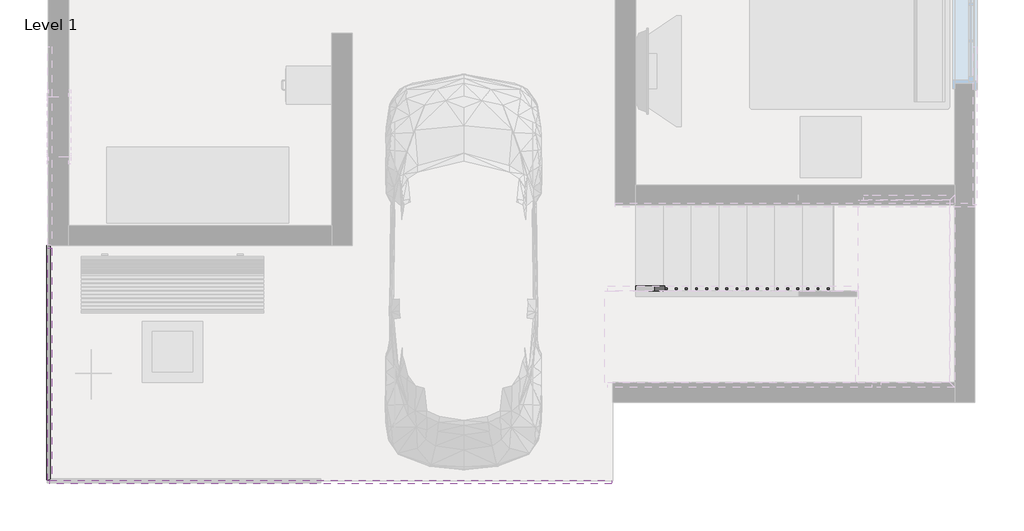
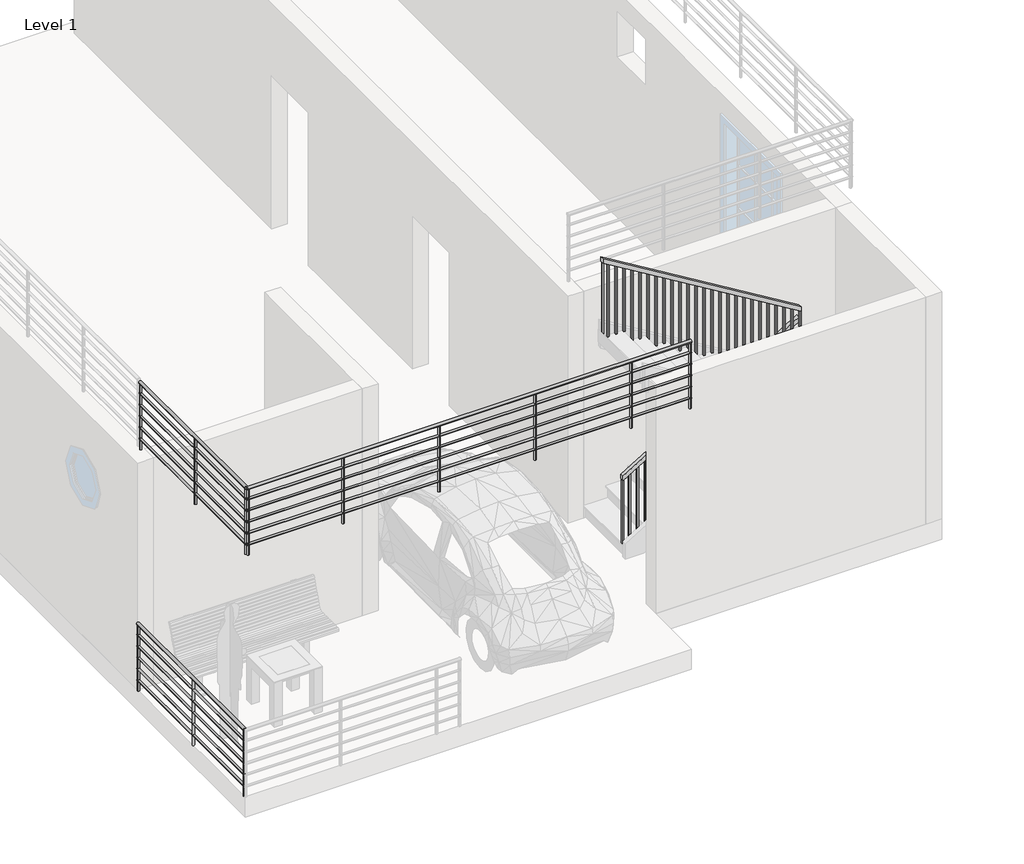
# One storey, part 2 of 4: 4 railings.
"""IFC4 building model written with IfcOpenShell, lengths in millimetres."""

from ifc_helpers import new_model, si_unit, point, frame, frame_2d, origin, origin_with_axes, place, context, project, spatial, polyline, circle_curve, trimmed, segment, composite_curve, outline, extrude, element, save

model = new_model("IFC4")

# Units and contexts
model_context = context("Model", 3, world=origin())
ifc_project = project(units=[si_unit("LENGTHUNIT", "METRE", prefix="MILLI")], contexts=[model_context])

# Site, building, storey
site = spatial("IfcSite", under=ifc_project)
building = spatial("IfcBuilding", under=site)
storey = spatial("IfcBuildingStorey", under=building, Name="Level 1", Elevation=0.0)

# Railings
placement = place(None, origin())
element("IfcRailing", 1, ObjectType="Handrail - Pipe", at=placement, inside=storey, context=model_context, shape_type="SweptSolid", body=[
    extrude(outline(composite_curve([segment(trimmed(circle_curve(frame_2d((4146.55, -14409.9389568)), 19.05), [point((4146.55, -14428.9889568))], [point((4146.55, -14390.8889568))], False, "CARTESIAN"), True, "CONTINUOUS"), segment(trimmed(circle_curve(frame_2d((4146.55, -14409.9389568)), 19.05), [point((4146.55, -14390.8889568))], [point((4146.55, -14428.9889568))], False, "CARTESIAN"), True, "CONTINUOUS")], self_intersect=False)), frame((0.0, 1290.5342758, 0.0), z_axis=(0.0, 1.0, 0.0), x_axis=(0.0, 0.0, 1.0)), (0.0, 0.0, 1.0), 2336.8),
    extrude(outline(composite_curve([segment(trimmed(circle_curve(frame_2d((4000.5, -14409.9389568)), 12.7), [point((4000.5, -14397.2389568))], [point((4000.5, -14422.6389568))], False, "CARTESIAN"), True, "CONTINUOUS"), segment(trimmed(circle_curve(frame_2d((4000.5, -14409.9389568)), 12.7), [point((4000.5, -14422.6389568))], [point((4000.5, -14397.2389568))], False, "CARTESIAN"), True, "CONTINUOUS")], self_intersect=False)), frame((0.0, 1290.5342758, 0.0), z_axis=(0.0, 1.0, 0.0), x_axis=(0.0, 0.0, 1.0)), (0.0, 0.0, 1.0), 2336.8),
    extrude(outline(composite_curve([segment(trimmed(circle_curve(frame_2d((3848.1, -14409.9389568)), 12.7), [point((3848.1, -14397.2389568))], [point((3848.1, -14422.6389568))], False, "CARTESIAN"), True, "CONTINUOUS"), segment(trimmed(circle_curve(frame_2d((3848.1, -14409.9389568)), 12.7), [point((3848.1, -14422.6389568))], [point((3848.1, -14397.2389568))], False, "CARTESIAN"), True, "CONTINUOUS")], self_intersect=False)), frame((0.0, 1290.5342758, 0.0), z_axis=(0.0, 1.0, 0.0), x_axis=(0.0, 0.0, 1.0)), (0.0, 0.0, 1.0), 2336.8),
    extrude(outline(composite_curve([segment(trimmed(circle_curve(frame_2d((3695.7, -14409.9389568)), 12.7), [point((3695.7, -14397.2389568))], [point((3695.7, -14422.6389568))], False, "CARTESIAN"), True, "CONTINUOUS"), segment(trimmed(circle_curve(frame_2d((3695.7, -14409.9389568)), 12.7), [point((3695.7, -14422.6389568))], [point((3695.7, -14397.2389568))], False, "CARTESIAN"), True, "CONTINUOUS")], self_intersect=False)), frame((0.0, 1290.5342758, 0.0), z_axis=(0.0, 1.0, 0.0), x_axis=(0.0, 0.0, 1.0)), (0.0, 0.0, 1.0), 2336.8),
    extrude(outline(composite_curve([segment(trimmed(circle_curve(frame_2d((3543.3, -14409.9389568)), 12.7), [point((3543.3, -14397.2389568))], [point((3543.3, -14422.6389568))], False, "CARTESIAN"), True, "CONTINUOUS"), segment(trimmed(circle_curve(frame_2d((3543.3, -14409.9389568)), 12.7), [point((3543.3, -14422.6389568))], [point((3543.3, -14397.2389568))], False, "CARTESIAN"), True, "CONTINUOUS")], self_intersect=False)), frame((0.0, 1290.5342758, 0.0), z_axis=(0.0, 1.0, 0.0), x_axis=(0.0, 0.0, 1.0)), (0.0, 0.0, 1.0), 2336.8),
    extrude(outline(composite_curve([segment(trimmed(circle_curve(frame_2d((3390.9, -14409.9389568)), 12.7), [point((3390.9, -14397.2389568))], [point((3390.9, -14422.6389568))], False, "CARTESIAN"), True, "CONTINUOUS"), segment(trimmed(circle_curve(frame_2d((3390.9, -14409.9389568)), 12.7), [point((3390.9, -14422.6389568))], [point((3390.9, -14397.2389568))], False, "CARTESIAN"), True, "CONTINUOUS")], self_intersect=False)), frame((0.0, 1290.5342758, 0.0), z_axis=(0.0, 1.0, 0.0), x_axis=(0.0, 0.0, 1.0)), (0.0, 0.0, 1.0), 2336.8),
    extrude(outline(composite_curve([segment(trimmed(circle_curve(frame_2d((-14409.9389568, 2408.1342758)), 12.7), [point((-14397.2389568, 2408.1342758))], [point((-14422.6389568, 2408.1342758))], False, "CARTESIAN"), True, "CONTINUOUS"), segment(trimmed(circle_curve(frame_2d((-14409.9389568, 2408.1342758)), 12.7), [point((-14422.6389568, 2408.1342758))], [point((-14397.2389568, 2408.1342758))], False, "CARTESIAN"), True, "CONTINUOUS")], self_intersect=False)), frame((0.0, 0.0, 3251.2), z_axis=(0.0, 0.0, 1.0), x_axis=(1.0, 0.0, 0.0)), (0.0, 0.0, 1.0), 876.3),
    extrude(outline(composite_curve([segment(trimmed(circle_curve(frame_2d((-14409.9389568, 1303.2342758)), 12.7), [point((-14397.2389568, 1303.2342758))], [point((-14422.6389568, 1303.2342758))], False, "CARTESIAN"), True, "CONTINUOUS"), segment(trimmed(circle_curve(frame_2d((-14409.9389568, 1303.2342758)), 12.7), [point((-14422.6389568, 1303.2342758))], [point((-14397.2389568, 1303.2342758))], False, "CARTESIAN"), True, "CONTINUOUS")], self_intersect=False)), frame((0.0, 0.0, 3251.2), z_axis=(0.0, 0.0, 1.0), x_axis=(1.0, 0.0, 0.0)), (0.0, 0.0, 1.0), 876.3),
    extrude(outline(composite_curve([segment(trimmed(circle_curve(frame_2d((-14409.9389568, 3614.6342758)), 12.7), [point((-14397.2389568, 3614.6342758))], [point((-14422.6389568, 3614.6342758))], False, "CARTESIAN"), True, "CONTINUOUS"), segment(trimmed(circle_curve(frame_2d((-14409.9389568, 3614.6342758)), 12.7), [point((-14422.6389568, 3614.6342758))], [point((-14397.2389568, 3614.6342758))], False, "CARTESIAN"), True, "CONTINUOUS")], self_intersect=False)), frame((0.0, 0.0, 3251.2), z_axis=(0.0, 0.0, 1.0), x_axis=(1.0, 0.0, 0.0)), (0.0, 0.0, 1.0), 876.3),
])
element("IfcRailing", 2, ObjectType="Handrail - Pipe", at=placement, inside=storey, context=model_context, shape_type="SweptSolid", body=[
    extrude(outline(composite_curve([segment(trimmed(circle_curve(frame_2d((895.35, -14422.6389568)), 19.05), [point((895.35, -14441.6889568))], [point((895.35, -14403.5889568))], False, "CARTESIAN"), True, "CONTINUOUS"), segment(trimmed(circle_curve(frame_2d((895.35, -14422.6389568)), 19.05), [point((895.35, -14403.5889568))], [point((895.35, -14441.6889568))], False, "CARTESIAN"), True, "CONTINUOUS")], self_intersect=False)), frame((0.0, 1303.2342758, 0.0), z_axis=(0.0, 1.0, 0.0), x_axis=(0.0, 0.0, 1.0)), (0.0, 0.0, 1.0), 2349.5),
    extrude(outline(composite_curve([segment(trimmed(circle_curve(frame_2d((749.3, -14422.6389568)), 12.7), [point((749.3, -14409.9389568))], [point((749.3, -14435.3389568))], False, "CARTESIAN"), True, "CONTINUOUS"), segment(trimmed(circle_curve(frame_2d((749.3, -14422.6389568)), 12.7), [point((749.3, -14435.3389568))], [point((749.3, -14409.9389568))], False, "CARTESIAN"), True, "CONTINUOUS")], self_intersect=False)), frame((0.0, 1303.2342758, 0.0), z_axis=(0.0, 1.0, 0.0), x_axis=(0.0, 0.0, 1.0)), (0.0, 0.0, 1.0), 2349.5),
    extrude(outline(composite_curve([segment(trimmed(circle_curve(frame_2d((596.9, -14422.6389568)), 12.7), [point((596.9, -14409.9389568))], [point((596.9, -14435.3389568))], False, "CARTESIAN"), True, "CONTINUOUS"), segment(trimmed(circle_curve(frame_2d((596.9, -14422.6389568)), 12.7), [point((596.9, -14435.3389568))], [point((596.9, -14409.9389568))], False, "CARTESIAN"), True, "CONTINUOUS")], self_intersect=False)), frame((0.0, 1303.2342758, 0.0), z_axis=(0.0, 1.0, 0.0), x_axis=(0.0, 0.0, 1.0)), (0.0, 0.0, 1.0), 2349.5),
    extrude(outline(composite_curve([segment(trimmed(circle_curve(frame_2d((444.5, -14422.6389568)), 12.7), [point((444.5, -14409.9389568))], [point((444.5, -14435.3389568))], False, "CARTESIAN"), True, "CONTINUOUS"), segment(trimmed(circle_curve(frame_2d((444.5, -14422.6389568)), 12.7), [point((444.5, -14435.3389568))], [point((444.5, -14409.9389568))], False, "CARTESIAN"), True, "CONTINUOUS")], self_intersect=False)), frame((0.0, 1303.2342758, 0.0), z_axis=(0.0, 1.0, 0.0), x_axis=(0.0, 0.0, 1.0)), (0.0, 0.0, 1.0), 2349.5),
    extrude(outline(composite_curve([segment(trimmed(circle_curve(frame_2d((292.1, -14422.6389568)), 12.7), [point((292.1, -14409.9389568))], [point((292.1, -14435.3389568))], False, "CARTESIAN"), True, "CONTINUOUS"), segment(trimmed(circle_curve(frame_2d((292.1, -14422.6389568)), 12.7), [point((292.1, -14435.3389568))], [point((292.1, -14409.9389568))], False, "CARTESIAN"), True, "CONTINUOUS")], self_intersect=False)), frame((0.0, 1303.2342758, 0.0), z_axis=(0.0, 1.0, 0.0), x_axis=(0.0, 0.0, 1.0)), (0.0, 0.0, 1.0), 2349.5),
    extrude(outline(composite_curve([segment(trimmed(circle_curve(frame_2d((139.7, -14422.6389568)), 12.7), [point((139.7, -14409.9389568))], [point((139.7, -14435.3389568))], False, "CARTESIAN"), True, "CONTINUOUS"), segment(trimmed(circle_curve(frame_2d((139.7, -14422.6389568)), 12.7), [point((139.7, -14435.3389568))], [point((139.7, -14409.9389568))], False, "CARTESIAN"), True, "CONTINUOUS")], self_intersect=False)), frame((0.0, 1303.2342758, 0.0), z_axis=(0.0, 1.0, 0.0), x_axis=(0.0, 0.0, 1.0)), (0.0, 0.0, 1.0), 2349.5),
    extrude(outline(composite_curve([segment(trimmed(circle_curve(frame_2d((-14422.6389568, 2433.5342758)), 12.7), [point((-14409.9389568, 2433.5342758))], [point((-14435.3389568, 2433.5342758))], False, "CARTESIAN"), True, "CONTINUOUS"), segment(trimmed(circle_curve(frame_2d((-14422.6389568, 2433.5342758)), 12.7), [point((-14435.3389568, 2433.5342758))], [point((-14409.9389568, 2433.5342758))], False, "CARTESIAN"), True, "CONTINUOUS")], self_intersect=False)), origin_with_axes(), (0.0, 0.0, 1.0), 876.3),
    extrude(outline(composite_curve([segment(trimmed(circle_curve(frame_2d((-14422.6389568, 1315.9342758)), 12.7), [point((-14409.9389568, 1315.9342758))], [point((-14435.3389568, 1315.9342758))], False, "CARTESIAN"), True, "CONTINUOUS"), segment(trimmed(circle_curve(frame_2d((-14422.6389568, 1315.9342758)), 12.7), [point((-14435.3389568, 1315.9342758))], [point((-14409.9389568, 1315.9342758))], False, "CARTESIAN"), True, "CONTINUOUS")], self_intersect=False)), origin_with_axes(), (0.0, 0.0, 1.0), 876.3),
    extrude(outline(composite_curve([segment(trimmed(circle_curve(frame_2d((-14422.6389568, 3640.0342758)), 12.7), [point((-14409.9389568, 3640.0342758))], [point((-14435.3389568, 3640.0342758))], False, "CARTESIAN"), True, "CONTINUOUS"), segment(trimmed(circle_curve(frame_2d((-14422.6389568, 3640.0342758)), 12.7), [point((-14435.3389568, 3640.0342758))], [point((-14409.9389568, 3640.0342758))], False, "CARTESIAN"), True, "CONTINUOUS")], self_intersect=False)), origin_with_axes(), (0.0, 0.0, 1.0), 876.3),
])
element("IfcRailing", 3, ObjectType="Handrail - Pipe", at=placement, inside=storey, context=model_context, shape_type="SweptSolid", body=[
    extrude(outline(composite_curve([segment(trimmed(circle_curve(frame_2d((1277.8342758, 4146.55)), 19.05), [point((1258.7842758, 4146.55))], [point((1296.8842758, 4146.55))], False, "CARTESIAN"), True, "CONTINUOUS"), segment(trimmed(circle_curve(frame_2d((1277.8342758, 4146.55)), 19.05), [point((1296.8842758, 4146.55))], [point((1258.7842758, 4146.55))], False, "CARTESIAN"), True, "CONTINUOUS")], self_intersect=False)), frame((-14409.9389568, 0.0, 0.0), z_axis=(1.0, 0.0, 0.0), x_axis=(0.0, 1.0, 0.0)), (0.0, 0.0, 1.0), 5638.8),
    extrude(outline(composite_curve([segment(trimmed(circle_curve(frame_2d((1277.8342758, 4000.5)), 12.7), [point((1290.5342758, 4000.5))], [point((1265.1342758, 4000.5))], False, "CARTESIAN"), True, "CONTINUOUS"), segment(trimmed(circle_curve(frame_2d((1277.8342758, 4000.5)), 12.7), [point((1265.1342758, 4000.5))], [point((1290.5342758, 4000.5))], False, "CARTESIAN"), True, "CONTINUOUS")], self_intersect=False)), frame((-14409.9389568, 0.0, 0.0), z_axis=(1.0, 0.0, 0.0), x_axis=(0.0, 1.0, 0.0)), (0.0, 0.0, 1.0), 5638.8),
    extrude(outline(composite_curve([segment(trimmed(circle_curve(frame_2d((1277.8342758, 3848.1)), 12.7), [point((1290.5342758, 3848.1))], [point((1265.1342758, 3848.1))], False, "CARTESIAN"), True, "CONTINUOUS"), segment(trimmed(circle_curve(frame_2d((1277.8342758, 3848.1)), 12.7), [point((1265.1342758, 3848.1))], [point((1290.5342758, 3848.1))], False, "CARTESIAN"), True, "CONTINUOUS")], self_intersect=False)), frame((-14409.9389568, 0.0, 0.0), z_axis=(1.0, 0.0, 0.0), x_axis=(0.0, 1.0, 0.0)), (0.0, 0.0, 1.0), 5638.8),
    extrude(outline(composite_curve([segment(trimmed(circle_curve(frame_2d((1277.8342758, 3695.7)), 12.7), [point((1290.5342758, 3695.7))], [point((1265.1342758, 3695.7))], False, "CARTESIAN"), True, "CONTINUOUS"), segment(trimmed(circle_curve(frame_2d((1277.8342758, 3695.7)), 12.7), [point((1265.1342758, 3695.7))], [point((1290.5342758, 3695.7))], False, "CARTESIAN"), True, "CONTINUOUS")], self_intersect=False)), frame((-14409.9389568, 0.0, 0.0), z_axis=(1.0, 0.0, 0.0), x_axis=(0.0, 1.0, 0.0)), (0.0, 0.0, 1.0), 5638.8),
    extrude(outline(composite_curve([segment(trimmed(circle_curve(frame_2d((1277.8342758, 3543.3)), 12.7), [point((1290.5342758, 3543.3))], [point((1265.1342758, 3543.3))], False, "CARTESIAN"), True, "CONTINUOUS"), segment(trimmed(circle_curve(frame_2d((1277.8342758, 3543.3)), 12.7), [point((1265.1342758, 3543.3))], [point((1290.5342758, 3543.3))], False, "CARTESIAN"), True, "CONTINUOUS")], self_intersect=False)), frame((-14409.9389568, 0.0, 0.0), z_axis=(1.0, 0.0, 0.0), x_axis=(0.0, 1.0, 0.0)), (0.0, 0.0, 1.0), 5638.8),
    extrude(outline(composite_curve([segment(trimmed(circle_curve(frame_2d((1277.8342758, 3390.9)), 12.7), [point((1290.5342758, 3390.9))], [point((1265.1342758, 3390.9))], False, "CARTESIAN"), True, "CONTINUOUS"), segment(trimmed(circle_curve(frame_2d((1277.8342758, 3390.9)), 12.7), [point((1265.1342758, 3390.9))], [point((1290.5342758, 3390.9))], False, "CARTESIAN"), True, "CONTINUOUS")], self_intersect=False)), frame((-14409.9389568, 0.0, 0.0), z_axis=(1.0, 0.0, 0.0), x_axis=(0.0, 1.0, 0.0)), (0.0, 0.0, 1.0), 5638.8),
    extrude(outline(composite_curve([segment(trimmed(circle_curve(frame_2d((-9533.1389568, 1277.8342758)), 12.7), [point((-9533.1389568, 1290.5342758))], [point((-9533.1389568, 1265.1342758))], False, "CARTESIAN"), True, "CONTINUOUS"), segment(trimmed(circle_curve(frame_2d((-9533.1389568, 1277.8342758)), 12.7), [point((-9533.1389568, 1265.1342758))], [point((-9533.1389568, 1290.5342758))], False, "CARTESIAN"), True, "CONTINUOUS")], self_intersect=False)), frame((0.0, 0.0, 3251.2), z_axis=(0.0, 0.0, 1.0), x_axis=(1.0, 0.0, 0.0)), (0.0, 0.0, 1.0), 876.3),
    extrude(outline(composite_curve([segment(trimmed(circle_curve(frame_2d((-10752.3389568, 1277.8342758)), 12.7), [point((-10752.3389568, 1290.5342758))], [point((-10752.3389568, 1265.1342758))], False, "CARTESIAN"), True, "CONTINUOUS"), segment(trimmed(circle_curve(frame_2d((-10752.3389568, 1277.8342758)), 12.7), [point((-10752.3389568, 1265.1342758))], [point((-10752.3389568, 1290.5342758))], False, "CARTESIAN"), True, "CONTINUOUS")], self_intersect=False)), frame((0.0, 0.0, 3251.2), z_axis=(0.0, 0.0, 1.0), x_axis=(1.0, 0.0, 0.0)), (0.0, 0.0, 1.0), 876.3),
    extrude(outline(composite_curve([segment(trimmed(circle_curve(frame_2d((-11971.5389568, 1277.8342758)), 12.7), [point((-11971.5389568, 1290.5342758))], [point((-11971.5389568, 1265.1342758))], False, "CARTESIAN"), True, "CONTINUOUS"), segment(trimmed(circle_curve(frame_2d((-11971.5389568, 1277.8342758)), 12.7), [point((-11971.5389568, 1265.1342758))], [point((-11971.5389568, 1290.5342758))], False, "CARTESIAN"), True, "CONTINUOUS")], self_intersect=False)), frame((0.0, 0.0, 3251.2), z_axis=(0.0, 0.0, 1.0), x_axis=(1.0, 0.0, 0.0)), (0.0, 0.0, 1.0), 876.3),
    extrude(outline(composite_curve([segment(trimmed(circle_curve(frame_2d((-13190.7389568, 1277.8342758)), 12.7), [point((-13190.7389568, 1290.5342758))], [point((-13190.7389568, 1265.1342758))], False, "CARTESIAN"), True, "CONTINUOUS"), segment(trimmed(circle_curve(frame_2d((-13190.7389568, 1277.8342758)), 12.7), [point((-13190.7389568, 1265.1342758))], [point((-13190.7389568, 1290.5342758))], False, "CARTESIAN"), True, "CONTINUOUS")], self_intersect=False)), frame((0.0, 0.0, 3251.2), z_axis=(0.0, 0.0, 1.0), x_axis=(1.0, 0.0, 0.0)), (0.0, 0.0, 1.0), 876.3),
    extrude(outline(composite_curve([segment(trimmed(circle_curve(frame_2d((-8783.8389568, 1277.8342758)), 12.7), [point((-8783.8389568, 1290.5342758))], [point((-8783.8389568, 1265.1342758))], False, "CARTESIAN"), True, "CONTINUOUS"), segment(trimmed(circle_curve(frame_2d((-8783.8389568, 1277.8342758)), 12.7), [point((-8783.8389568, 1265.1342758))], [point((-8783.8389568, 1290.5342758))], False, "CARTESIAN"), True, "CONTINUOUS")], self_intersect=False)), frame((0.0, 0.0, 3251.2), z_axis=(0.0, 0.0, 1.0), x_axis=(1.0, 0.0, 0.0)), (0.0, 0.0, 1.0), 876.3),
    extrude(outline(composite_curve([segment(trimmed(circle_curve(frame_2d((-14397.2389568, 1277.8342758)), 12.7), [point((-14397.2389568, 1290.5342758))], [point((-14397.2389568, 1265.1342758))], False, "CARTESIAN"), True, "CONTINUOUS"), segment(trimmed(circle_curve(frame_2d((-14397.2389568, 1277.8342758)), 12.7), [point((-14397.2389568, 1265.1342758))], [point((-14397.2389568, 1290.5342758))], False, "CARTESIAN"), True, "CONTINUOUS")], self_intersect=False)), frame((0.0, 0.0, 3251.2), z_axis=(0.0, 0.0, 1.0), x_axis=(1.0, 0.0, 0.0)), (0.0, 0.0, 1.0), 876.3),
])
element("IfcRailing", 4, ObjectType="Handrail - Rectangular", at=placement, inside=storey, context=model_context, shape_type="SweptSolid", body=[
    extrude(outline(polyline([(1083.7333333, -8529.8389568), (1024.3318731, -8529.8389568), (2378.9985397, -6294.6389568), (2438.4, -6294.6389568), (1083.7333333, -8529.8389568)])), frame((0.0, 3195.5342758, 0.0), z_axis=(0.0, 1.0, 0.0), x_axis=(0.0, 0.0, 1.0)), (0.0, 0.0, 1.0), 50.8),
    extrude(outline(polyline([(2548.3318731, -6294.6389568), (2607.7333333, -6294.6389568), (4131.7333333, -8809.2389568), (4072.3318731, -8809.2389568), (2548.3318731, -6294.6389568)])), frame((0.0, 3144.7342758, 0.0), z_axis=(0.0, 1.0, 0.0), x_axis=(0.0, 0.0, 1.0)), (0.0, 0.0, 1.0), 50.8),
    extrude(outline(polyline([(4020.3773276, -8723.5139568), (4031.9227822, -8742.5639568), (3048.0, -8742.5639568), (3048.0, -8723.5139568), (4020.3773276, -8723.5139568)])), frame((0.0, 3160.6092758, 0.0), z_axis=(0.0, 1.0, 0.0), x_axis=(0.0, 0.0, 1.0)), (0.0, 0.0, 1.0), 19.05),
    extrude(outline(polyline([(3958.80157, -8621.9139568), (3970.3470246, -8640.9639568), (3048.0, -8640.9639568), (3048.0, -8621.9139568), (3958.80157, -8621.9139568)])), frame((0.0, 3160.6092758, 0.0), z_axis=(0.0, 1.0, 0.0), x_axis=(0.0, 0.0, 1.0)), (0.0, 0.0, 1.0), 19.05),
    extrude(outline(polyline([(3897.2258125, -8520.3139568), (3908.771267, -8539.3639568), (3048.0, -8539.3639568), (3048.0, -8520.3139568), (3897.2258125, -8520.3139568)])), frame((0.0, 3160.6092758, 0.0), z_axis=(0.0, 1.0, 0.0), x_axis=(0.0, 0.0, 1.0)), (0.0, 0.0, 1.0), 19.05),
    extrude(outline(polyline([(3835.6500549, -8418.7139568), (3847.1955094, -8437.7639568), (2878.6666667, -8437.7639568), (2878.6666667, -8418.7139568), (3835.6500549, -8418.7139568)])), frame((0.0, 3160.6092758, 0.0), z_axis=(0.0, 1.0, 0.0), x_axis=(0.0, 0.0, 1.0)), (0.0, 0.0, 1.0), 19.05),
    extrude(outline(polyline([(3774.0742973, -8317.1139568), (3785.6197519, -8336.1639568), (2878.6666667, -8336.1639568), (2878.6666667, -8317.1139568), (3774.0742973, -8317.1139568)])), frame((0.0, 3160.6092758, 0.0), z_axis=(0.0, 1.0, 0.0), x_axis=(0.0, 0.0, 1.0)), (0.0, 0.0, 1.0), 19.05),
    extrude(outline(polyline([(3712.4985397, -8215.5139568), (3724.0439943, -8234.5639568), (2709.3333333, -8234.5639568), (2709.3333333, -8215.5139568), (3712.4985397, -8215.5139568)])), frame((0.0, 3160.6092758, 0.0), z_axis=(0.0, 1.0, 0.0), x_axis=(0.0, 0.0, 1.0)), (0.0, 0.0, 1.0), 19.05),
    extrude(outline(polyline([(3650.9227822, -8113.9139568), (3662.4682367, -8132.9639568), (2709.3333333, -8132.9639568), (2709.3333333, -8113.9139568), (3650.9227822, -8113.9139568)])), frame((0.0, 3160.6092758, 0.0), z_axis=(0.0, 1.0, 0.0), x_axis=(0.0, 0.0, 1.0)), (0.0, 0.0, 1.0), 19.05),
    extrude(outline(polyline([(3589.3470246, -8012.3139568), (3600.8924791, -8031.3639568), (2709.3333333, -8031.3639568), (2709.3333333, -8012.3139568), (3589.3470246, -8012.3139568)])), frame((0.0, 3160.6092758, 0.0), z_axis=(0.0, 1.0, 0.0), x_axis=(0.0, 0.0, 1.0)), (0.0, 0.0, 1.0), 19.05),
    extrude(outline(polyline([(3527.771267, -7910.7139568), (3539.3167216, -7929.7639568), (2540.0, -7929.7639568), (2540.0, -7910.7139568), (3527.771267, -7910.7139568)])), frame((0.0, 3160.6092758, 0.0), z_axis=(0.0, 1.0, 0.0), x_axis=(0.0, 0.0, 1.0)), (0.0, 0.0, 1.0), 19.05),
    extrude(outline(polyline([(3466.1955094, -7809.1139568), (3477.740964, -7828.1639568), (2540.0, -7828.1639568), (2540.0, -7809.1139568), (3466.1955094, -7809.1139568)])), frame((0.0, 3160.6092758, 0.0), z_axis=(0.0, 1.0, 0.0), x_axis=(0.0, 0.0, 1.0)), (0.0, 0.0, 1.0), 19.05),
    extrude(outline(polyline([(3404.6197519, -7707.5139568), (3416.1652064, -7726.5639568), (2540.0, -7726.5639568), (2540.0, -7707.5139568), (3404.6197519, -7707.5139568)])), frame((0.0, 3160.6092758, 0.0), z_axis=(0.0, 1.0, 0.0), x_axis=(0.0, 0.0, 1.0)), (0.0, 0.0, 1.0), 19.05),
    extrude(outline(polyline([(3343.0439943, -7605.9139568), (3354.5894488, -7624.9639568), (2370.6666667, -7624.9639568), (2370.6666667, -7605.9139568), (3343.0439943, -7605.9139568)])), frame((0.0, 3160.6092758, 0.0), z_axis=(0.0, 1.0, 0.0), x_axis=(0.0, 0.0, 1.0)), (0.0, 0.0, 1.0), 19.05),
    extrude(outline(polyline([(3281.4682367, -7504.3139568), (3293.0136913, -7523.3639568), (2370.6666667, -7523.3639568), (2370.6666667, -7504.3139568), (3281.4682367, -7504.3139568)])), frame((0.0, 3160.6092758, 0.0), z_axis=(0.0, 1.0, 0.0), x_axis=(0.0, 0.0, 1.0)), (0.0, 0.0, 1.0), 19.05),
    extrude(outline(polyline([(3219.8924791, -7402.7139568), (3231.4379337, -7421.7639568), (2370.6666667, -7421.7639568), (2370.6666667, -7402.7139568), (3219.8924791, -7402.7139568)])), frame((0.0, 3160.6092758, 0.0), z_axis=(0.0, 1.0, 0.0), x_axis=(0.0, 0.0, 1.0)), (0.0, 0.0, 1.0), 19.05),
    extrude(outline(polyline([(3158.3167216, -7301.1139568), (3169.8621761, -7320.1639568), (2201.3333333, -7320.1639568), (2201.3333333, -7301.1139568), (3158.3167216, -7301.1139568)])), frame((0.0, 3160.6092758, 0.0), z_axis=(0.0, 1.0, 0.0), x_axis=(0.0, 0.0, 1.0)), (0.0, 0.0, 1.0), 19.05),
    extrude(outline(polyline([(3096.740964, -7199.5139568), (3108.2864185, -7218.5639568), (2201.3333333, -7218.5639568), (2201.3333333, -7199.5139568), (3096.740964, -7199.5139568)])), frame((0.0, 3160.6092758, 0.0), z_axis=(0.0, 1.0, 0.0), x_axis=(0.0, 0.0, 1.0)), (0.0, 0.0, 1.0), 19.05),
    extrude(outline(polyline([(3035.1652064, -7097.9139568), (3046.710661, -7116.9639568), (2032.0, -7116.9639568), (2032.0, -7097.9139568), (3035.1652064, -7097.9139568)])), frame((0.0, 3160.6092758, 0.0), z_axis=(0.0, 1.0, 0.0), x_axis=(0.0, 0.0, 1.0)), (0.0, 0.0, 1.0), 19.05),
    extrude(outline(polyline([(2973.5894488, -6996.3139568), (2985.1349034, -7015.3639568), (2032.0, -7015.3639568), (2032.0, -6996.3139568), (2973.5894488, -6996.3139568)])), frame((0.0, 3160.6092758, 0.0), z_axis=(0.0, 1.0, 0.0), x_axis=(0.0, 0.0, 1.0)), (0.0, 0.0, 1.0), 19.05),
    extrude(outline(polyline([(2912.0136913, -6894.7139568), (2923.5591458, -6913.7639568), (2032.0, -6913.7639568), (2032.0, -6894.7139568), (2912.0136913, -6894.7139568)])), frame((0.0, 3160.6092758, 0.0), z_axis=(0.0, 1.0, 0.0), x_axis=(0.0, 0.0, 1.0)), (0.0, 0.0, 1.0), 19.05),
    extrude(outline(polyline([(2850.4379337, -6793.1139568), (2861.9833882, -6812.1639568), (1862.6666667, -6812.1639568), (1862.6666667, -6793.1139568), (2850.4379337, -6793.1139568)])), frame((0.0, 3160.6092758, 0.0), z_axis=(0.0, 1.0, 0.0), x_axis=(0.0, 0.0, 1.0)), (0.0, 0.0, 1.0), 19.05),
    extrude(outline(polyline([(2788.8621761, -6691.5139568), (2800.4076307, -6710.5639568), (1862.6666667, -6710.5639568), (1862.6666667, -6691.5139568), (2788.8621761, -6691.5139568)])), frame((0.0, 3160.6092758, 0.0), z_axis=(0.0, 1.0, 0.0), x_axis=(0.0, 0.0, 1.0)), (0.0, 0.0, 1.0), 19.05),
    extrude(outline(polyline([(2727.2864185, -6589.9139568), (2738.8318731, -6608.9639568), (1862.6666667, -6608.9639568), (1862.6666667, -6589.9139568), (2727.2864185, -6589.9139568)])), frame((0.0, 3160.6092758, 0.0), z_axis=(0.0, 1.0, 0.0), x_axis=(0.0, 0.0, 1.0)), (0.0, 0.0, 1.0), 19.05),
    extrude(outline(polyline([(2665.710661, -6488.3139568), (2677.2561155, -6507.3639568), (1693.3333333, -6507.3639568), (1693.3333333, -6488.3139568), (2665.710661, -6488.3139568)])), frame((0.0, 3160.6092758, 0.0), z_axis=(0.0, 1.0, 0.0), x_axis=(0.0, 0.0, 1.0)), (0.0, 0.0, 1.0), 19.05),
    extrude(outline(polyline([(2604.1349034, -6386.7139568), (2615.6803579, -6405.7639568), (1693.3333333, -6405.7639568), (1693.3333333, -6386.7139568), (2604.1349034, -6386.7139568)])), frame((0.0, 3160.6092758, 0.0), z_axis=(0.0, 1.0, 0.0), x_axis=(0.0, 0.0, 1.0)), (0.0, 0.0, 1.0), 19.05),
    extrude(outline(polyline([(2323.1955094, -6386.7139568), (2311.6500549, -6405.7639568), (1354.6666667, -6405.7639568), (1354.6666667, -6386.7139568), (2323.1955094, -6386.7139568)])), frame((0.0, 3211.4092758, 0.0), z_axis=(0.0, 1.0, 0.0), x_axis=(0.0, 0.0, 1.0)), (0.0, 0.0, 1.0), 19.05),
    extrude(outline(polyline([(2261.6197519, -6488.3139568), (2250.0742973, -6507.3639568), (1354.6666667, -6507.3639568), (1354.6666667, -6488.3139568), (2261.6197519, -6488.3139568)])), frame((0.0, 3211.4092758, 0.0), z_axis=(0.0, 1.0, 0.0), x_axis=(0.0, 0.0, 1.0)), (0.0, 0.0, 1.0), 19.05),
    extrude(outline(polyline([(2200.0439943, -6589.9139568), (2188.4985397, -6608.9639568), (1185.3333333, -6608.9639568), (1185.3333333, -6589.9139568), (2200.0439943, -6589.9139568)])), frame((0.0, 3211.4092758, 0.0), z_axis=(0.0, 1.0, 0.0), x_axis=(0.0, 0.0, 1.0)), (0.0, 0.0, 1.0), 19.05),
    extrude(outline(polyline([(2138.4682367, -6691.5139568), (2126.9227822, -6710.5639568), (1185.3333333, -6710.5639568), (1185.3333333, -6691.5139568), (2138.4682367, -6691.5139568)])), frame((0.0, 3211.4092758, 0.0), z_axis=(0.0, 1.0, 0.0), x_axis=(0.0, 0.0, 1.0)), (0.0, 0.0, 1.0), 19.05),
    extrude(outline(polyline([(2076.8924791, -6793.1139568), (2065.3470246, -6812.1639568), (1185.3333333, -6812.1639568), (1185.3333333, -6793.1139568), (2076.8924791, -6793.1139568)])), frame((0.0, 3211.4092758, 0.0), z_axis=(0.0, 1.0, 0.0), x_axis=(0.0, 0.0, 1.0)), (0.0, 0.0, 1.0), 19.05),
    extrude(outline(polyline([(2015.3167216, -6894.7139568), (2003.771267, -6913.7639568), (1016.0, -6913.7639568), (1016.0, -6894.7139568), (2015.3167216, -6894.7139568)])), frame((0.0, 3211.4092758, 0.0), z_axis=(0.0, 1.0, 0.0), x_axis=(0.0, 0.0, 1.0)), (0.0, 0.0, 1.0), 19.05),
    extrude(outline(polyline([(1953.740964, -6996.3139568), (1942.1955094, -7015.3639568), (1016.0, -7015.3639568), (1016.0, -6996.3139568), (1953.740964, -6996.3139568)])), frame((0.0, 3211.4092758, 0.0), z_axis=(0.0, 1.0, 0.0), x_axis=(0.0, 0.0, 1.0)), (0.0, 0.0, 1.0), 19.05),
    extrude(outline(polyline([(1892.1652064, -7097.9139568), (1880.6197519, -7116.9639568), (1016.0, -7116.9639568), (1016.0, -7097.9139568), (1892.1652064, -7097.9139568)])), frame((0.0, 3211.4092758, 0.0), z_axis=(0.0, 1.0, 0.0), x_axis=(0.0, 0.0, 1.0)), (0.0, 0.0, 1.0), 19.05),
    extrude(outline(polyline([(1830.5894488, -7199.5139568), (1819.0439943, -7218.5639568), (846.6666667, -7218.5639568), (846.6666667, -7199.5139568), (1830.5894488, -7199.5139568)])), frame((0.0, 3211.4092758, 0.0), z_axis=(0.0, 1.0, 0.0), x_axis=(0.0, 0.0, 1.0)), (0.0, 0.0, 1.0), 19.05),
    extrude(outline(polyline([(1769.0136913, -7301.1139568), (1757.4682367, -7320.1639568), (846.6666667, -7320.1639568), (846.6666667, -7301.1139568), (1769.0136913, -7301.1139568)])), frame((0.0, 3211.4092758, 0.0), z_axis=(0.0, 1.0, 0.0), x_axis=(0.0, 0.0, 1.0)), (0.0, 0.0, 1.0), 19.05),
    extrude(outline(polyline([(1707.4379337, -7402.7139568), (1695.8924791, -7421.7639568), (846.6666667, -7421.7639568), (846.6666667, -7402.7139568), (1707.4379337, -7402.7139568)])), frame((0.0, 3211.4092758, 0.0), z_axis=(0.0, 1.0, 0.0), x_axis=(0.0, 0.0, 1.0)), (0.0, 0.0, 1.0), 19.05),
    extrude(outline(polyline([(1645.8621761, -7504.3139568), (1634.3167216, -7523.3639568), (677.3333333, -7523.3639568), (677.3333333, -7504.3139568), (1645.8621761, -7504.3139568)])), frame((0.0, 3211.4092758, 0.0), z_axis=(0.0, 1.0, 0.0), x_axis=(0.0, 0.0, 1.0)), (0.0, 0.0, 1.0), 19.05),
    extrude(outline(polyline([(1584.2864185, -7605.9139568), (1572.740964, -7624.9639568), (677.3333333, -7624.9639568), (677.3333333, -7605.9139568), (1584.2864185, -7605.9139568)])), frame((0.0, 3211.4092758, 0.0), z_axis=(0.0, 1.0, 0.0), x_axis=(0.0, 0.0, 1.0)), (0.0, 0.0, 1.0), 19.05),
    extrude(outline(polyline([(1522.710661, -7707.5139568), (1511.1652064, -7726.5639568), (508.0, -7726.5639568), (508.0, -7707.5139568), (1522.710661, -7707.5139568)])), frame((0.0, 3211.4092758, 0.0), z_axis=(0.0, 1.0, 0.0), x_axis=(0.0, 0.0, 1.0)), (0.0, 0.0, 1.0), 19.05),
    extrude(outline(polyline([(1461.1349034, -7809.1139568), (1449.5894488, -7828.1639568), (508.0, -7828.1639568), (508.0, -7809.1139568), (1461.1349034, -7809.1139568)])), frame((0.0, 3211.4092758, 0.0), z_axis=(0.0, 1.0, 0.0), x_axis=(0.0, 0.0, 1.0)), (0.0, 0.0, 1.0), 19.05),
    extrude(outline(polyline([(1399.5591458, -7910.7139568), (1388.0136913, -7929.7639568), (508.0, -7929.7639568), (508.0, -7910.7139568), (1399.5591458, -7910.7139568)])), frame((0.0, 3211.4092758, 0.0), z_axis=(0.0, 1.0, 0.0), x_axis=(0.0, 0.0, 1.0)), (0.0, 0.0, 1.0), 19.05),
    extrude(outline(polyline([(1337.9833882, -8012.3139568), (1326.4379337, -8031.3639568), (338.6666667, -8031.3639568), (338.6666667, -8012.3139568), (1337.9833882, -8012.3139568)])), frame((0.0, 3211.4092758, 0.0), z_axis=(0.0, 1.0, 0.0), x_axis=(0.0, 0.0, 1.0)), (0.0, 0.0, 1.0), 19.05),
    extrude(outline(polyline([(1276.4076307, -8113.9139568), (1264.8621761, -8132.9639568), (338.6666667, -8132.9639568), (338.6666667, -8113.9139568), (1276.4076307, -8113.9139568)])), frame((0.0, 3211.4092758, 0.0), z_axis=(0.0, 1.0, 0.0), x_axis=(0.0, 0.0, 1.0)), (0.0, 0.0, 1.0), 19.05),
    extrude(outline(polyline([(1214.8318731, -8215.5139568), (1203.2864185, -8234.5639568), (338.6666667, -8234.5639568), (338.6666667, -8215.5139568), (1214.8318731, -8215.5139568)])), frame((0.0, 3211.4092758, 0.0), z_axis=(0.0, 1.0, 0.0), x_axis=(0.0, 0.0, 1.0)), (0.0, 0.0, 1.0), 19.05),
    extrude(outline(polyline([(1153.2561155, -8317.1139568), (1141.710661, -8336.1639568), (169.3333333, -8336.1639568), (169.3333333, -8317.1139568), (1153.2561155, -8317.1139568)])), frame((0.0, 3211.4092758, 0.0), z_axis=(0.0, 1.0, 0.0), x_axis=(0.0, 0.0, 1.0)), (0.0, 0.0, 1.0), 19.05),
    extrude(outline(polyline([(1091.6803579, -8418.7139568), (1080.1349034, -8437.7639568), (169.3333333, -8437.7639568), (169.3333333, -8418.7139568), (1091.6803579, -8418.7139568)])), frame((0.0, 3211.4092758, 0.0), z_axis=(0.0, 1.0, 0.0), x_axis=(0.0, 0.0, 1.0)), (0.0, 0.0, 1.0), 19.05),
    extrude(outline(polyline([(2542.5591458, -6285.1139568), (2554.1046004, -6304.1639568), (1693.3333333, -6304.1639568), (1693.3333333, -6285.1139568), (2542.5591458, -6285.1139568)])), frame((0.0, 3160.6092758, 0.0), z_axis=(0.0, 1.0, 0.0), x_axis=(0.0, 0.0, 1.0)), (0.0, 0.0, 1.0), 19.05),
    extrude(outline(polyline([(4060.7864185, -8790.1889568), (4072.3318731, -8809.2389568), (3048.0, -8809.2389568), (3048.0, -8790.1889568), (4060.7864185, -8790.1889568)])), frame((0.0, 3160.6092758, 0.0), z_axis=(0.0, 1.0, 0.0), x_axis=(0.0, 0.0, 1.0)), (0.0, 0.0, 1.0), 19.05),
    extrude(outline(polyline([(1035.8773276, -8510.7889568), (1024.3318731, -8529.8389568), (169.3333333, -8529.8389568), (169.3333333, -8510.7889568), (1035.8773276, -8510.7889568)])), frame((0.0, 3211.4092758, 0.0), z_axis=(0.0, 1.0, 0.0), x_axis=(0.0, 0.0, 1.0)), (0.0, 0.0, 1.0), 19.05),
])

save(model, "model.ifc")

# Revit data of these elements
# Type "Handrail - Pipe"
#   Assembly Code = "C2010400"
#   built-in parameter 1008612 = 0.0416667 (stored number, unit not read)
#   built-in parameter 1008611 = 0.0833333 (stored number, unit not read)
#   built-in parameter 1008609 = 4 (stored number, unit not read)
#   built-in parameter 1008604 = 0.166667 (stored number, unit not read)
#   built-in parameter 1008603 = 0.166667 (stored number, unit not read)
#   Railing Height = 3' - 0"
#   built-in parameter 1008630 = 2
#   built-in parameter 1008610 = 1
#   built-in parameter 1008605 = 1
#   built-in parameter 1008618 = Baluster - Round : 1"
# Type "Handrail - Rectangular"
#   Assembly Code = "C2010400"
#   built-in parameter 1008612 = 0.0416667 (stored number, unit not read)
#   built-in parameter 1008611 = 0.0416667 (stored number, unit not read)
#   built-in parameter 1008609 = 0.333333 (stored number, unit not read)
#   built-in parameter 1008604 = 0.166667 (stored number, unit not read)
#   built-in parameter 1008603 = 0.166667 (stored number, unit not read)
#   Railing Height = 3' - 0"
#   built-in parameter 1008630 = 2
#   built-in parameter 1008610 = 2
#   built-in parameter 1008618 = Baluster - Square : 3/4"
# Elements 1, 3 (IfcRailing, "Handrail - Pipe")
#   built-in parameter 1008621 = 10.6667 (stored number, unit not read)
#   Phase Created = New Construction
# Element 2 (IfcRailing, "Handrail - Pipe")
#   Phase Created = New Construction
# Element 4 (IfcRailing, "Handrail - Rectangular")
#   Phase Created = New Construction
